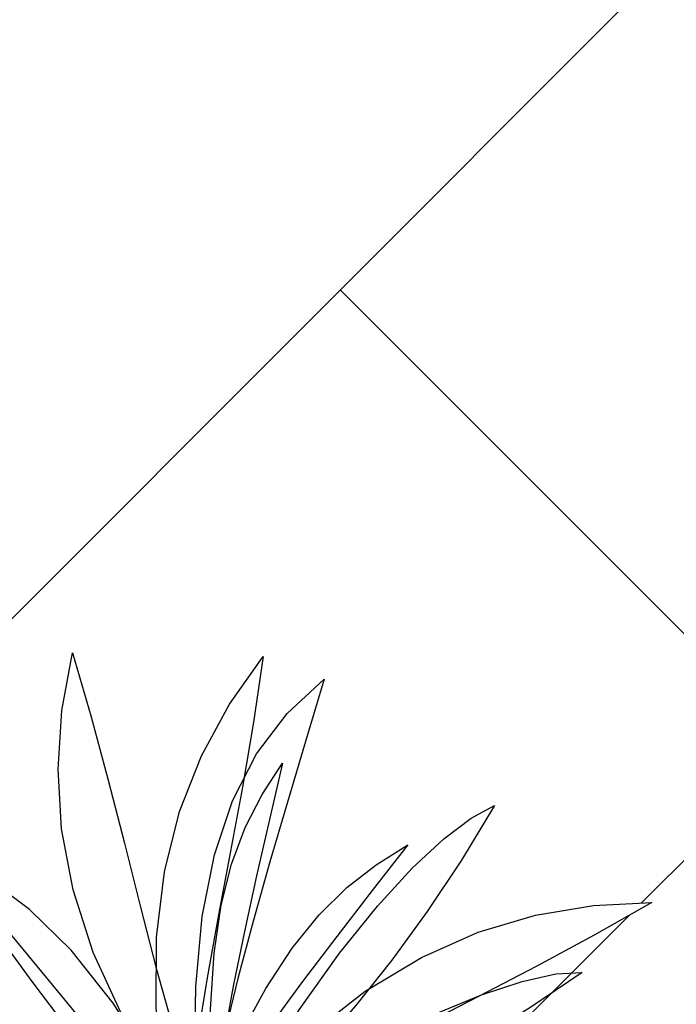
# Model space of a CAD drawing. Units: inches. Extents: x 3590 to 5167, y 65 to 1917.
# Tile 34 of 100: x 4947 to 4968, y 1357 to 1388. Entities that reach past the tile are written whole.
import ezdxf

# ---------------------------------------------------------------- set-up
doc = ezdxf.new("R2010")
doc.units = ezdxf.units.IN
doc.layers.add('A-FLOR-PATT', color=8, linetype='Continuous', lineweight=13)
doc.layers.add('L-PLNT', color=94, linetype='Continuous', lineweight=18)
doc.layers.add('DIENHOA', color=3, linetype='Continuous')

# ---------------------------------------------------------------- blocks, each defined once
blk = doc.blocks.new('Cay03_mb')
at = {"layer": 'DIENHOA'}
for p, q in [((118.6, 555.3), (166.2, 599.1)), ((166.2, 599.1), (142.2, 519.4)), ((79.5, 503.7), (118.6, 555.3)), ((142.2, 519.4), (119, 441.7)), ((48.6, 443.6), (79.5, 503.7)), ((25.5, 374.3), (48.6, 443.6)), ((119, 441.7), (96.7, 365.6)), ((9.9, 295.3), (25.5, 374.3)), ((96.7, 365.6), (75.6, 290.6)), ((-211.2, 304.6), (-263.5, 343.5)), ((-158, 252.3), (-211.2, 304.6)), ((436.8, 297.2), (511, 309.6)), ((511, 309.6), (585.9, 313.5)), ((585.9, 313.5), (511.8, 271.4)), ((1.6, 205.7), (9.9, 295.3)), ((75.6, 290.6), (55.7, 216.3)), ((363.4, 275.4), (436.8, 297.2)), ((-240.2, 277.8), (-88.4, 94.9)), ((290.6, 243.2), (363.4, 275.4)), ((511.8, 271.4), (437.6, 231.5)), ((-104.2, 184.4), (-158, 252.3)), ((218.5, 199.8), (290.6, 243.2)), ((437.6, 231.5), (363.7, 192.9)), ((55.7, 216.3), (37.3, 142.1)), ((0.2, 104.9), (1.6, 205.7)), ((147, 144.1), (218.5, 199.8)), ((363.7, 192.9), (290.2, 154.9)), ((-49.6, 98.5), (-104.2, 184.4))]:
    blk.add_line(p, q, dxfattribs=at)
for points in [[(23.7, -5.4), (-41, 82.2), (-91.8, 167.1), (-129.7, 249.5), (-155.6, 329.6), (-170.2, 407.8), (-174.7, 484.2), (-169.8, 559.3), (-156.5, 633.1)], [(-156.5, 633.1), (-132.5, 551.3), (-110.5, 470), (-89.8, 389.2), (-69.6, 309), (-49, 229.4), (-27.1, 150.4), (-3.2, 72.1), (23.7, -5.4)], [(-16.4, -26.7), (-38.3, 80), (-48.9, 178.3), (-48.7, 269), (-38.5, 352.6), (-19.1, 429.7), (9, 501), (44.9, 567.1), (87.9, 628.5)], [(87.9, 628.5), (75.5, 544.2), (61.3, 461.2), (46.1, 379.1), (30.8, 297.8), (16.1, 216.9), (2.9, 136), (-8.3, 54.9), (-16.4, -26.7)], [(23.7, -5.4), (19.8, 93), (20.3, 177), (25, 248.5), (34, 309.8), (47.3, 362.7), (64.9, 409.3), (86.8, 451.7), (112.9, 491.9)], [(112.9, 491.9), (96, 419.7), (79.5, 347.4), (63.9, 276.5), (50, 208.4), (38.4, 144.8), (29.7, 86.9), (24.6, 36.3), (23.7, -5.4)], [(-395.6, 473.7), (-347.5, 405.6), (-300.6, 339.5), (-254.3, 275.1), (-208.3, 212.3), (-161.9, 150.9), (-114.8, 90.7), (-66.5, 31.6), (-16.4, -26.7)], [(384.3, 437.5), (342.2, 367.8), (298.1, 301.7), (252.6, 239.4), (206.1, 181.1), (159.4, 127.2), (113, 78), (67.6, 33.6), (23.7, -5.4)], [(23.7, -5.4), (79.9, 91.7), (134.1, 176.2), (185.8, 248.4), (234.3, 308.7), (279, 357.3), (319.3, 394.8), (354.6, 421.4), (384.3, 437.5)], [(273.2, 387.3), (227.6, 328.8), (182.3, 270.1), (138.4, 212.3), (97.2, 156.4), (60, 103.4), (27.8, 54.6), (1.9, 10.8), (-16.4, -26.7)], [(-16.4, -26.7), (21.4, 64.2), (57, 140.3), (91.4, 203.3), (125.2, 255.1), (159.5, 297.5), (195, 332.5), (232.7, 361.8), (273.2, 387.3)], [(496.7, 224), (429.4, 178.4), (361.6, 136.9), (294.1, 99.5), (227.5, 66.1), (162.4, 36.7), (99.7, 11.5), (39.8, -9.7), (-16.4, -26.7)], [(-16.4, -26.7), (75.4, 37.9), (160.1, 91.8), (237.3, 135.7), (306.6, 170), (367.6, 195.4), (419.9, 212.5), (463.1, 221.9), (496.7, 224)]]:
    blk.add_lwpolyline(points, dxfattribs=at)

msp = doc.modelspace()

# ---------------------------------------------------------------- hatches: boundary and pattern name
at = {"layer": 'A-FLOR-PATT', "transparency": 33554687}
h = msp.add_hatch(dxfattribs=at)
h.set_pattern_fill('AR-HBONE', color=256, scale=0.2)
h.set_pattern_definition([(45, (-588.972, 0), (0, 28.73682), [60.96, -20.32]), (135, (-574.604, 14.368), (3e-15, 28.73682), [60.96, -20.32])])
h.paths.add_polyline_path([(5071.274, 1796.999), (4933.274, 1796.999), (4933.274, 1753.999), (4962.774, 1753.999, -0.414214), (4928.774, 1719.999), (4933.274, 1718.999), (4933.274, 1334.999), (5071.274, 1334.999)])
h.paths.add_polyline_path([(4951.78, 1521.077), (4951.715, 1521.04), (4951.563, 1520.895)], flags=16)
h.paths.add_polyline_path([(4952.267, 1521.376), (4952.198, 1521.371), (4952.198, 1521.356)], flags=0)
h.paths.add_polyline_path([(4967.051, 1529.728), (4965.231, 1528.694), (4963.411, 1527.714), (4961.756, 1526.851), (4963.589, 1527.449), (4964.036, 1527.478), (4962.975, 1527.249), (4961.76, 1526.852), (4959.792, 1525.834), (4958.005, 1524.895), (4956.24, 1523.93), (4954.504, 1522.919), (4954.129, 1522.682), (4953.361, 1521.997), (4953.366, 1521.998), (4953.605, 1522.064), (4955.106, 1522.761), (4956.921, 1523.434), (4958.678, 1523.915), (4960.358, 1524.2), (4961.945, 1524.286), (4964.171, 1524.108), (4965.958, 1523.309), (4963.863, 1522.976), (4965.187, 1522.499), (4963.366, 1522.497), (4961.545, 1522.487), (4959.764, 1522.461), (4958.304, 1522.419), (4957.974, 1522.388), (4956.307, 1522.232), (4954.718, 1522.071), (4953.251, 1521.899), (4953.525, 1521.623), (4954.331, 1521.379), (4956.243, 1521.23), (4958.039, 1520.93), (4959.684, 1520.483), (4961.16, 1519.896), (4963.107, 1518.8), (4964.393, 1517.325), (4962.973, 1517.726), (4964.558, 1516.661), (4965.407, 1515.708), (4963.507, 1516.322), (4961.68, 1517.005), (4959.935, 1517.745), (4958.282, 1518.528), (4956.732, 1519.343), (4955.295, 1520.175), (4954.672, 1520.572), (4954.513, 1520.627), (4955.658, 1519.318), (4956.703, 1517.982), (4957.644, 1516.647), (4958.485, 1515.334), (4959.55, 1513.524), (4960.438, 1511.769), (4958.841, 1513.62), (4957.452, 1515.325), (4955.819, 1517.459), (4956.665, 1515.448), (4957.111, 1513.923), (4957.447, 1511.714), (4957.076, 1509.793), (4956.538, 1511.11), (4955.992, 1512.569), (4955.444, 1514.125), (4954.898, 1515.735), (4954.357, 1517.356), (4953.824, 1518.943), (4953.305, 1520.452), (4953.065, 1521.116), (4952.971, 1521.146), (4952.949, 1521.086), (4952.73, 1520.199), (4953.37, 1518.024), (4953.757, 1516.373), (4954.051, 1514.765), (4954.264, 1513.221), (4954.471, 1511.131), (4954.497, 1510.402), (4954.409, 1511.76), (4954.264, 1513.221), (4954.051, 1514.765), (4953.757, 1516.373), (4953.37, 1518.024), (4952.877, 1519.698), (4952.716, 1520.141), (4952.533, 1519.059), (4952.374, 1517.789), (4952.219, 1516.312), (4952.046, 1514.6), (4951.833, 1512.626), (4951.557, 1510.363), (4951.203, 1512.168), (4950.852, 1514.339), (4950.985, 1516.376), (4951.66, 1518.286), (4952.593, 1520.481), (4952.357, 1521.13), (4951.855, 1520.328), (4950.839, 1518.908), (4949.777, 1517.587), (4948.916, 1516.617), (4948.111, 1515.256), (4947.089, 1513.554), (4945.889, 1511.615), (4946.326, 1513.402), (4946.562, 1514.249), (4945.528, 1513.327), (4944.581, 1512.531), (4946.018, 1514.508), (4947.204, 1516.048), (4947.893, 1517.313), (4949.307, 1518.764), (4950.414, 1519.767), (4950.451, 1519.806), (4952.267, 1521.376), (4951.645, 1521.493), (4950.404, 1521.18), (4948.044, 1520.359), (4946.119, 1519.452), (4944.572, 1518.475), (4943.35, 1517.443), (4941.997, 1515.92), (4941.661, 1515.275), (4942.813, 1516.99), (4944.572, 1518.475), (4946.119, 1519.452), (4948.044, 1520.359), (4950.404, 1521.18), (4951.645, 1521.493), (4949.647, 1521.868), (4948.6, 1521.756), (4947.126, 1521.57), (4945.42, 1521.348), (4943.45, 1521.105), (4941.183, 1520.856), (4942.86, 1521.613), (4943.873, 1522.03), (4942.952, 1521.909), (4941.41, 1521.485), (4939.543, 1520.67), (4938.968, 1520.226), (4940.733, 1521.299), (4942.952, 1521.909), (4943.702, 1522.008), (4945.894, 1522.7), (4947.565, 1522.714), (4948.921, 1522.566), (4951.131, 1522.183), (4950.971, 1522.297), (4948.129, 1523.006), (4946.035, 1523.707), (4944.232, 1524.521), (4942.707, 1525.461), (4941.444, 1526.537), (4940.43, 1527.761), (4939.649, 1529.143), (4941.421, 1528.122), (4943.147, 1527.132), (4944.841, 1526.175), (4946.514, 1525.25), (4948.179, 1524.359), (4948.365, 1524.263), (4946.475, 1526.045), (4945.181, 1527.54), (4944.19, 1529.033), (4943.496, 1530.54), (4943.278, 1531.36), (4942.498, 1531.919), (4943.114, 1531.762), (4942.959, 1533.659), (4944.14, 1531.989), (4944.612, 1531.323), (4946.202, 1530.463), (4947.486, 1529.509), (4948.79, 1528.226), (4950.368, 1526.237), (4949.485, 1528.155), (4948.851, 1530.123), (4948.491, 1532.041), (4948.381, 1533.918), (4948.501, 1535.76), (4948.827, 1537.573), (4949.418, 1535.565), (4949.957, 1533.569), (4950.464, 1531.586), (4950.961, 1529.617), (4951.391, 1527.954), (4951.724, 1530.687), (4952.201, 1532.58), (4952.889, 1534.33), (4953.77, 1535.951), (4954.827, 1537.46), (4954.521, 1535.39), (4954.273, 1533.937), (4955.58, 1535.663), (4956.748, 1536.739), (4956.159, 1534.78), (4955.589, 1532.873), (4955.043, 1531.006), (4954.525, 1529.166), (4954.038, 1527.341), (4953.638, 1525.733), (4953.611, 1525.586), (4953.398, 1524.166), (4953.382, 1524.009), (4954.07, 1525.476), (4954.912, 1527.022), (4956.136, 1528.894), (4957.847, 1530.577), (4959.376, 1531.54), (4958.256, 1530.104), (4957.143, 1528.663), (4956.066, 1527.243), (4955.056, 1525.871), (4954.141, 1524.571), (4953.352, 1523.372), (4953.311, 1523.303), (4953.273, 1522.925), (4953.261, 1522.382), (4954.103, 1523.373), (4954.63, 1524.284), (4955.961, 1526.358), (4957.23, 1528.13), (4958.421, 1529.609), (4960.037, 1531.368), (4961.374, 1532.375), (4962.101, 1532.77), (4961.07, 1531.061), (4959.987, 1529.438), (4958.869, 1527.908), (4958.15, 1527.007), (4959.803, 1528.003), (4961.589, 1528.793), (4963.391, 1529.328), (4965.211, 1529.632)], flags=16)
h.paths.add_polyline_path([(4962.944, 1523.182), (4961.107, 1523.422), (4960.392, 1523.362), (4962.35, 1523.331)], flags=0)
h.paths.add_polyline_path([(5049.541, 1584.551), (5049.476, 1584.515), (5049.325, 1584.37)], flags=16)
h.paths.add_polyline_path([(5050.028, 1584.851), (5049.959, 1584.845), (5049.959, 1584.83)], flags=0)
h.paths.add_polyline_path([(5042.333, 1581.949), (5043.88, 1582.926), (5045.806, 1583.833), (5048.165, 1584.654), (5049.406, 1584.967), (5047.408, 1585.342), (5046.361, 1585.231), (5044.888, 1585.044), (5043.181, 1584.822), (5041.211, 1584.579), (5038.944, 1584.33), (5040.622, 1585.087), (5041.634, 1585.504), (5040.713, 1585.383), (5039.171, 1584.959), (5037.304, 1584.144), (5036.729, 1583.7), (5038.494, 1584.773), (5040.713, 1585.383), (5041.463, 1585.482), (5043.655, 1586.174), (5045.326, 1586.188), (5046.682, 1586.04), (5048.893, 1585.657), (5048.732, 1585.771), (5045.891, 1586.48), (5043.796, 1587.181), (5041.994, 1587.996), (5040.468, 1588.935), (5039.205, 1590.011), (5038.191, 1591.235), (5037.41, 1592.617), (5039.182, 1591.596), (5040.909, 1590.607), (5042.602, 1589.649), (5044.275, 1588.724), (5045.94, 1587.833), (5046.126, 1587.738), (5044.237, 1589.519), (5042.942, 1591.015), (5041.952, 1592.508), (5041.257, 1594.014), (5041.039, 1594.834), (5040.26, 1595.393), (5040.875, 1595.237), (5040.721, 1597.133), (5041.901, 1595.463), (5042.373, 1594.798), (5043.963, 1593.938), (5045.247, 1592.983), (5046.552, 1591.701), (5048.129, 1589.712), (5047.247, 1591.63), (5046.613, 1593.597), (5046.252, 1595.515), (5046.142, 1597.392), (5046.262, 1599.234), (5046.588, 1601.047), (5047.179, 1599.039), (5047.718, 1597.043), (5048.225, 1595.06), (5048.722, 1593.091), (5049.152, 1591.429), (5049.485, 1594.161), (5049.962, 1596.054), (5050.65, 1597.804), (5051.532, 1599.425), (5052.589, 1600.934), (5052.283, 1598.864), (5052.034, 1597.411), (5053.341, 1599.137), (5054.509, 1600.213), (5053.92, 1598.254), (5053.35, 1596.348), (5052.805, 1594.48), (5052.286, 1592.64), (5051.799, 1590.815), (5051.4, 1589.207), (5051.373, 1589.06), (5051.159, 1587.64), (5051.143, 1587.483), (5051.831, 1588.95), (5052.673, 1590.496), (5053.898, 1592.368), (5055.608, 1594.051), (5057.137, 1595.014), (5056.017, 1593.578), (5054.904, 1592.137), (5053.828, 1590.717), (5052.817, 1589.345), (5051.902, 1588.046), (5051.113, 1586.846), (5051.072, 1586.777), (5051.034, 1586.399), (5051.022, 1585.856), (5051.864, 1586.847), (5052.391, 1587.758), (5053.723, 1589.832), (5054.991, 1591.604), (5056.182, 1593.083), (5057.798, 1594.842), (5059.135, 1595.849), (5059.863, 1596.244), (5058.831, 1594.535), (5057.749, 1592.912), (5056.63, 1591.382), (5055.912, 1590.482), (5057.564, 1591.477), (5059.35, 1592.267), (5061.152, 1592.802), (5062.972, 1593.106), (5064.812, 1593.203), (5062.992, 1592.169), (5061.172, 1591.188), (5059.518, 1590.325), (5061.35, 1590.924), (5061.797, 1590.952), (5060.737, 1590.723), (5059.521, 1590.326), (5057.553, 1589.308), (5055.766, 1588.369), (5054.002, 1587.404), (5052.265, 1586.393), (5051.891, 1586.156), (5051.122, 1585.471), (5051.127, 1585.472), (5051.366, 1585.538), (5052.867, 1586.235), (5054.682, 1586.908), (5056.439, 1587.389), (5058.12, 1587.675), (5059.706, 1587.76), (5061.933, 1587.583), (5063.719, 1586.783), (5061.624, 1586.45), (5062.949, 1585.973), (5061.127, 1585.971), (5059.307, 1585.961), (5057.525, 1585.935), (5056.065, 1585.893), (5055.735, 1585.862), (5054.068, 1585.707), (5052.479, 1585.546), (5051.012, 1585.373), (5051.286, 1585.097), (5052.092, 1584.853), (5054.004, 1584.704), (5055.8, 1584.404), (5057.446, 1583.958), (5058.921, 1583.37), (5060.868, 1582.274), (5062.154, 1580.799), (5060.734, 1581.2), (5062.32, 1580.135), (5063.168, 1579.182), (5061.269, 1579.796), (5059.441, 1580.479), (5057.696, 1581.219), (5056.043, 1582.003), (5054.493, 1582.817), (5053.057, 1583.649), (5052.433, 1584.047), (5052.274, 1584.101), (5053.42, 1582.793), (5054.464, 1581.457), (5055.405, 1580.121), (5056.247, 1578.809), (5057.311, 1576.998), (5058.199, 1575.244), (5056.602, 1577.094), (5055.213, 1578.799), (5053.58, 1580.933), (5054.427, 1578.922), (5054.872, 1577.397), (5055.208, 1575.189), (5054.838, 1573.267), (5054.299, 1574.584), (5053.754, 1576.043), (5053.206, 1577.599), (5052.659, 1579.209), (5052.118, 1580.83), (5051.585, 1582.417), (5051.066, 1583.927), (5050.826, 1584.59), (5050.733, 1584.62), (5050.711, 1584.561), (5050.491, 1583.673), (5051.131, 1581.498), (5051.518, 1579.847), (5051.813, 1578.24), (5052.026, 1576.695), (5052.233, 1574.605), (5052.258, 1573.876), (5052.17, 1575.234), (5052.026, 1576.695), (5051.813, 1578.24), (5051.518, 1579.847), (5051.131, 1581.498), (5050.638, 1583.172), (5050.477, 1583.615), (5050.294, 1582.533), (5050.136, 1581.263), (5049.981, 1579.786), (5049.807, 1578.074), (5049.594, 1576.1), (5049.318, 1573.837), (5048.965, 1575.642), (5048.613, 1577.813), (5048.747, 1579.85), (5049.421, 1581.76), (5050.354, 1583.955), (5050.118, 1584.604), (5049.616, 1583.802), (5048.6, 1582.382), (5047.538, 1581.061), (5046.677, 1580.091), (5045.872, 1578.73), (5044.85, 1577.028), (5043.651, 1575.089), (5044.087, 1576.877), (5044.324, 1577.723), (5043.289, 1576.801), (5042.342, 1576.005), (5043.779, 1577.982), (5044.966, 1579.522), (5045.655, 1580.787), (5047.068, 1582.239), (5048.175, 1583.241), (5048.213, 1583.28), (5050.028, 1584.851), (5049.406, 1584.967), (5048.165, 1584.654), (5045.806, 1583.833), (5043.88, 1582.926), (5042.333, 1581.949), (5041.111, 1580.917), (5039.758, 1579.394), (5039.423, 1578.749), (5040.575, 1580.464)], flags=16)
h.paths.add_polyline_path([(4954.799, 1533.12), (4954.262, 1532.079), (4953.831, 1530.935), (4953.505, 1529.636), (4953.283, 1528.133), (4953.167, 1526.376), (4953.156, 1524.315), (4953.277, 1521.236), (4952.802, 1521.842), (4951.557, 1521.998), (4950.976, 1521.961), (4952.661, 1521.941), (4952.802, 1521.842), (4953.152, 1523.593), (4953.167, 1526.376), (4953.283, 1528.133), (4953.609, 1530.346), (4954.456, 1532.592)], flags=0)
h.paths.add_polyline_path([(5050.563, 1585.316), (5049.318, 1585.472), (5048.737, 1585.435), (5050.422, 1585.415), (5050.563, 1585.316), (5050.914, 1587.067), (5050.928, 1589.851), (5051.045, 1591.607), (5051.371, 1593.82), (5052.217, 1596.066), (5052.56, 1596.594), (5052.024, 1595.554), (5051.592, 1594.409), (5051.266, 1593.11), (5051.045, 1591.607), (5050.928, 1589.851), (5050.918, 1587.789), (5051.038, 1584.71)], flags=0)
h.paths.add_polyline_path([(5058.153, 1586.836), (5060.111, 1586.805), (5060.705, 1586.656), (5058.868, 1586.896)], flags=0)
h.paths.add_polyline_path([(5049.541, 1430.936), (5049.476, 1430.9), (5049.325, 1430.755)], flags=16)
h.paths.add_polyline_path([(5050.028, 1431.236), (5049.959, 1431.231), (5049.959, 1431.215)], flags=0)
h.paths.add_polyline_path([(5046.588, 1447.432), (5047.179, 1445.425), (5047.718, 1443.429), (5048.225, 1441.446), (5048.722, 1439.476), (5049.152, 1437.814), (5049.485, 1440.546), (5049.962, 1442.439), (5050.65, 1444.189), (5051.532, 1445.811), (5052.589, 1447.319), (5052.283, 1445.249), (5052.034, 1443.796), (5053.341, 1445.522), (5054.509, 1446.598), (5053.92, 1444.64), (5053.35, 1442.733), (5052.805, 1440.865), (5052.286, 1439.025), (5051.799, 1437.201), (5051.4, 1435.592), (5051.373, 1435.445), (5051.159, 1434.025), (5051.143, 1433.868), (5051.831, 1435.335), (5052.673, 1436.881), (5053.898, 1438.753), (5055.608, 1440.436), (5057.137, 1441.4), (5056.017, 1439.963), (5054.904, 1438.522), (5053.828, 1437.102), (5052.817, 1435.73), (5051.902, 1434.431), (5051.113, 1433.231), (5051.072, 1433.162), (5051.034, 1432.784), (5051.022, 1432.242), (5051.864, 1433.232), (5052.391, 1434.143), (5053.723, 1436.217), (5054.991, 1437.989), (5056.182, 1439.468), (5057.798, 1441.227), (5059.135, 1442.235), (5059.863, 1442.629), (5058.831, 1440.921), (5057.749, 1439.298), (5056.63, 1437.767), (5055.912, 1436.867), (5057.564, 1437.863), (5059.35, 1438.652), (5061.152, 1439.187), (5062.972, 1439.491), (5064.812, 1439.588), (5062.992, 1438.554), (5061.172, 1437.573), (5059.518, 1436.71), (5061.35, 1437.309), (5061.797, 1437.337), (5060.737, 1437.108), (5059.521, 1436.711), (5057.553, 1435.693), (5055.766, 1434.754), (5054.002, 1433.789), (5052.265, 1432.778), (5051.891, 1432.541), (5051.122, 1431.856), (5051.127, 1431.857), (5051.366, 1431.923), (5052.867, 1432.62), (5054.682, 1433.293), (5056.439, 1433.775), (5058.12, 1434.06), (5059.706, 1434.145), (5061.933, 1433.968), (5063.719, 1433.168), (5061.624, 1432.835), (5062.949, 1432.358), (5061.127, 1432.357), (5059.307, 1432.346), (5057.525, 1432.32), (5056.065, 1432.278), (5055.735, 1432.248), (5054.068, 1432.092), (5052.479, 1431.931), (5051.012, 1431.759), (5051.286, 1431.482), (5052.092, 1431.238), (5054.004, 1431.089), (5055.8, 1430.789), (5057.446, 1430.343), (5058.921, 1429.755), (5060.868, 1428.66), (5062.154, 1427.185), (5060.734, 1427.585), (5062.32, 1426.52), (5063.168, 1425.567), (5061.269, 1426.181), (5059.441, 1426.865), (5057.696, 1427.604), (5056.043, 1428.388), (5054.493, 1429.202), (5053.057, 1430.034), (5052.433, 1430.432), (5052.274, 1430.487), (5053.42, 1429.178), (5054.464, 1427.842), (5055.405, 1426.506), (5056.247, 1425.194), (5057.311, 1423.383), (5058.199, 1421.629), (5056.602, 1423.479), (5055.213, 1425.184), (5053.58, 1427.318), (5054.427, 1425.307), (5054.872, 1423.782), (5055.208, 1421.574), (5054.838, 1419.652), (5054.299, 1420.97), (5053.754, 1422.428), (5053.206, 1423.984), (5052.659, 1425.595), (5052.118, 1427.215), (5051.585, 1428.802), (5051.066, 1430.312), (5050.826, 1430.975), (5050.733, 1431.005), (5050.711, 1430.946), (5050.491, 1430.058), (5051.131, 1427.883), (5051.518, 1426.232), (5051.813, 1424.625), (5052.026, 1423.081), (5052.233, 1420.991), (5052.258, 1420.261), (5052.17, 1421.619), (5052.026, 1423.081), (5051.813, 1424.625), (5051.518, 1426.232), (5051.131, 1427.883), (5050.638, 1429.558), (5050.477, 1430.001), (5050.294, 1428.918), (5050.136, 1427.648), (5049.981, 1426.171), (5049.807, 1424.459), (5049.594, 1422.485), (5049.318, 1420.222), (5048.965, 1422.028), (5048.613, 1424.199), (5048.747, 1426.235), (5049.421, 1428.146), (5050.354, 1430.34), (5050.118, 1430.989), (5049.616, 1430.187), (5048.6, 1428.768), (5047.538, 1427.446), (5046.677, 1426.477), (5045.872, 1425.116), (5044.85, 1423.413), (5043.651, 1421.474), (5044.087, 1423.262), (5044.324, 1424.109), (5043.289, 1423.186), (5042.342, 1422.391), (5043.779, 1424.368), (5044.966, 1425.907), (5045.655, 1427.173), (5047.068, 1428.624), (5048.175, 1429.627), (5048.213, 1429.666), (5050.028, 1431.236), (5049.406, 1431.353), (5048.165, 1431.039), (5045.806, 1430.218), (5043.88, 1429.311), (5042.333, 1428.334), (5041.111, 1427.302), (5039.758, 1425.779), (5039.423, 1425.134), (5040.575, 1426.849), (5042.333, 1428.334), (5043.88, 1429.311), (5045.806, 1430.218), (5048.165, 1431.039), (5049.406, 1431.353), (5047.408, 1431.727), (5046.361, 1431.616), (5044.888, 1431.429), (5043.181, 1431.207), (5041.211, 1430.964), (5038.944, 1430.715), (5040.622, 1431.472), (5041.634, 1431.89), (5040.713, 1431.769), (5039.171, 1431.345), (5037.304, 1430.53), (5036.729, 1430.085), (5038.494, 1431.158), (5040.713, 1431.769), (5041.463, 1431.867), (5043.655, 1432.559), (5045.326, 1432.573), (5046.682, 1432.425), (5048.893, 1432.042), (5048.732, 1432.156), (5045.891, 1432.865), (5043.796, 1433.566), (5041.994, 1434.381), (5040.468, 1435.321), (5039.205, 1436.396), (5038.191, 1437.62), (5037.41, 1439.002), (5039.182, 1437.982), (5040.909, 1436.992), (5042.602, 1436.034), (5044.275, 1435.109), (5045.94, 1434.218), (5046.126, 1434.123), (5044.237, 1435.904), (5042.942, 1437.4), (5041.952, 1438.893), (5041.257, 1440.399), (5041.039, 1441.219), (5040.26, 1441.778), (5040.875, 1441.622), (5040.721, 1443.518), (5041.901, 1441.848), (5042.373, 1441.183), (5043.963, 1440.323), (5045.247, 1439.369), (5046.552, 1438.086), (5048.129, 1436.097), (5047.247, 1438.015), (5046.613, 1439.982), (5046.252, 1441.901), (5046.142, 1443.778), (5046.262, 1445.619)], flags=16)
h.paths.add_polyline_path([(5052.382, 1444.255), (5051.623, 1442.78), (5052.024, 1441.939), (5052.56, 1442.98)], flags=0)
h.paths.add_polyline_path([(5050.563, 1431.701), (5049.318, 1431.857), (5048.737, 1431.821), (5050.422, 1431.8)], flags=0)
h.paths.add_polyline_path([(5058.153, 1433.221), (5060.111, 1433.19), (5060.705, 1433.041), (5058.868, 1433.281)], flags=0)
h.paths.add_polyline_path([(5049.541, 1352.285), (5049.476, 1352.249), (5049.325, 1352.104)], flags=16)
h.paths.add_polyline_path([(5050.028, 1352.585), (5049.959, 1352.58), (5049.959, 1352.564)], flags=0)
h.paths.add_polyline_path([(5046.588, 1368.781), (5047.179, 1366.774), (5047.718, 1364.778), (5048.225, 1362.795), (5048.722, 1360.825), (5049.152, 1359.163), (5049.485, 1361.896), (5049.962, 1363.789), (5050.65, 1365.538), (5051.532, 1367.16), (5052.589, 1368.669), (5052.283, 1366.598), (5052.034, 1365.145), (5053.341, 1366.871), (5054.509, 1367.947), (5053.92, 1365.989), (5053.35, 1364.082), (5052.805, 1362.214), (5052.286, 1360.374), (5051.799, 1358.55), (5051.4, 1356.942), (5051.373, 1356.794), (5051.159, 1355.374), (5051.143, 1355.218), (5051.831, 1356.684), (5052.673, 1358.23), (5053.898, 1360.102), (5055.608, 1361.786), (5057.137, 1362.749), (5056.017, 1361.313), (5054.904, 1359.872), (5053.828, 1358.452), (5052.817, 1357.079), (5051.902, 1355.78), (5051.113, 1354.581), (5051.072, 1354.512), (5051.034, 1354.133), (5051.022, 1353.591), (5051.864, 1354.581), (5052.391, 1355.492), (5053.723, 1357.566), (5054.991, 1359.338), (5056.182, 1360.817), (5057.798, 1362.577), (5059.135, 1363.584), (5059.863, 1363.979), (5058.831, 1362.27), (5057.749, 1360.647), (5056.63, 1359.117), (5055.912, 1358.216), (5057.564, 1359.212), (5059.35, 1360.001), (5061.152, 1360.536), (5062.972, 1360.841), (5064.812, 1360.937), (5062.992, 1359.903), (5061.172, 1358.923), (5059.518, 1358.059), (5061.35, 1358.658), (5061.797, 1358.687), (5060.737, 1358.458), (5059.521, 1358.061), (5057.553, 1357.043), (5055.766, 1356.103), (5054.002, 1355.138), (5052.265, 1354.127), (5051.891, 1353.89), (5051.122, 1353.206), (5051.127, 1353.206), (5051.366, 1353.272), (5052.867, 1353.969), (5054.682, 1354.643), (5056.439, 1355.124), (5058.12, 1355.409), (5059.706, 1355.495), (5061.933, 1355.317), (5063.719, 1354.518), (5061.624, 1354.184), (5062.949, 1353.708), (5061.127, 1353.706), (5059.307, 1353.695), (5057.525, 1353.669), (5056.065, 1353.627), (5055.735, 1353.597), (5054.068, 1353.441), (5052.479, 1353.28), (5051.012, 1353.108), (5051.286, 1352.831), (5052.092, 1352.587), (5054.004, 1352.439), (5055.8, 1352.138), (5057.446, 1351.692), (5058.921, 1351.104), (5060.868, 1350.009), (5062.154, 1348.534), (5060.734, 1348.935), (5062.32, 1347.869), (5063.168, 1346.916), (5061.269, 1347.53), (5059.441, 1348.214), (5057.696, 1348.954), (5056.043, 1349.737), (5054.493, 1350.551), (5053.057, 1351.383), (5052.433, 1351.781), (5052.274, 1351.836), (5053.42, 1350.527), (5054.464, 1349.191), (5055.405, 1347.855), (5056.247, 1346.543), (5057.311, 1344.733), (5058.199, 1342.978), (5056.602, 1344.828), (5055.213, 1346.534), (5053.58, 1348.667), (5054.427, 1346.656), (5054.872, 1345.132), (5055.208, 1342.923), (5054.838, 1341.002), (5054.299, 1342.319), (5053.754, 1343.778), (5053.206, 1345.334), (5052.659, 1346.944), (5052.118, 1348.564), (5051.585, 1350.151), (5051.066, 1351.661), (5050.826, 1352.324), (5050.733, 1352.355), (5050.711, 1352.295), (5050.491, 1351.408), (5051.131, 1349.232), (5051.518, 1347.581), (5051.813, 1345.974), (5052.026, 1344.43), (5052.233, 1342.34), (5052.258, 1341.61), (5052.17, 1342.969), (5052.026, 1344.43), (5051.813, 1345.974), (5051.518, 1347.581), (5051.131, 1349.232), (5050.638, 1350.907), (5050.477, 1351.35), (5050.294, 1350.267), (5050.136, 1348.997), (5049.981, 1347.52), (5049.807, 1345.809), (5049.594, 1343.835), (5049.318, 1341.571), (5048.965, 1343.377), (5048.613, 1345.548), (5048.747, 1347.585), (5049.421, 1349.495), (5050.354, 1351.689), (5050.118, 1352.339), (5049.616, 1351.536), (5048.6, 1350.117), (5047.538, 1348.795), (5046.677, 1347.826), (5045.872, 1346.465), (5044.85, 1344.763), (5043.651, 1342.824), (5044.087, 1344.611), (5044.324, 1345.458), (5043.289, 1344.535), (5042.342, 1343.74), (5043.779, 1345.717), (5044.966, 1347.256), (5045.655, 1348.522), (5047.068, 1349.973), (5048.175, 1350.976), (5048.213, 1351.015), (5050.028, 1352.585), (5049.406, 1352.702), (5048.165, 1352.388), (5045.806, 1351.567), (5043.88, 1350.661), (5042.333, 1349.683), (5041.111, 1348.651), (5039.758, 1347.128), (5039.423, 1346.483), (5040.575, 1348.198), (5042.333, 1349.683), (5043.88, 1350.661), (5045.806, 1351.567), (5048.165, 1352.388), (5049.406, 1352.702), (5047.408, 1353.076), (5046.361, 1352.965), (5044.888, 1352.779), (5043.181, 1352.556), (5041.211, 1352.313), (5038.944, 1352.065), (5040.622, 1352.821), (5041.634, 1353.239), (5040.713, 1353.118), (5039.171, 1352.694), (5037.304, 1351.879), (5036.729, 1351.434), (5038.494, 1352.508), (5040.713, 1353.118), (5041.463, 1353.216), (5043.655, 1353.909), (5045.326, 1353.923), (5046.682, 1353.774), (5048.893, 1353.391), (5048.732, 1353.506), (5045.891, 1354.214), (5043.796, 1354.915), (5041.994, 1355.73), (5040.468, 1356.67), (5039.205, 1357.746), (5038.191, 1358.969), (5037.41, 1360.352), (5039.182, 1359.331), (5040.909, 1358.341), (5042.602, 1357.383), (5044.275, 1356.458), (5045.94, 1355.567), (5046.126, 1355.472), (5044.237, 1357.253), (5042.942, 1358.749), (5041.952, 1360.242), (5041.257, 1361.748), (5041.039, 1362.568), (5040.26, 1363.128), (5040.875, 1362.971), (5040.721, 1364.867), (5041.901, 1363.197), (5042.373, 1362.532), (5043.963, 1361.672), (5045.247, 1360.718), (5046.552, 1359.435), (5048.129, 1357.446), (5047.247, 1359.364), (5046.613, 1361.331), (5046.252, 1363.25), (5046.142, 1365.127), (5046.262, 1366.969)], flags=16)
h.paths.add_polyline_path([(5052.382, 1365.604), (5051.623, 1364.129), (5052.024, 1363.288), (5052.56, 1364.329)], flags=0)
h.paths.add_polyline_path([(4951.78, 1698.041), (4951.715, 1698.005), (4951.563, 1697.859)], flags=16)
h.paths.add_polyline_path([(4952.267, 1698.341), (4952.198, 1698.335), (4952.198, 1698.32)], flags=0)
h.paths.add_polyline_path([(4957.076, 1686.757), (4956.538, 1688.074), (4955.992, 1689.533), (4955.444, 1691.089), (4954.898, 1692.699), (4954.357, 1694.32), (4953.824, 1695.907), (4953.305, 1697.417), (4953.065, 1698.08), (4952.971, 1698.11), (4952.949, 1698.051), (4952.73, 1697.163), (4953.37, 1694.988), (4953.757, 1693.337), (4954.051, 1691.729), (4954.264, 1690.185), (4954.471, 1688.095), (4954.497, 1687.366), (4954.409, 1688.724), (4954.264, 1690.185), (4954.051, 1691.729), (4953.757, 1693.337), (4953.37, 1694.988), (4952.877, 1696.662), (4952.716, 1697.105), (4952.533, 1696.023), (4952.374, 1694.753), (4952.219, 1693.276), (4952.046, 1691.564), (4951.833, 1689.59), (4951.557, 1687.327), (4951.203, 1689.132), (4950.852, 1691.303), (4950.985, 1693.34), (4951.66, 1695.25), (4952.593, 1697.445), (4952.357, 1698.094), (4951.855, 1697.292), (4950.839, 1695.872), (4949.777, 1694.551), (4948.916, 1693.581), (4948.111, 1692.22), (4947.089, 1690.518), (4945.889, 1688.579), (4946.326, 1690.366), (4946.562, 1691.213), (4945.528, 1690.291), (4944.581, 1689.495), (4946.018, 1691.472), (4947.204, 1693.012), (4947.893, 1694.277), (4949.307, 1695.729), (4950.414, 1696.731), (4950.451, 1696.77), (4952.267, 1698.341), (4951.645, 1698.457), (4950.404, 1698.144), (4948.044, 1697.323), (4946.119, 1696.416), (4944.572, 1695.439), (4943.35, 1694.407), (4941.997, 1692.884), (4941.661, 1692.239), (4942.813, 1693.954), (4944.572, 1695.439), (4946.119, 1696.416), (4948.044, 1697.323), (4950.404, 1698.144), (4951.645, 1698.457), (4949.647, 1698.832), (4948.6, 1698.72), (4947.126, 1698.534), (4945.42, 1698.312), (4943.45, 1698.069), (4941.183, 1697.82), (4942.86, 1698.577), (4943.873, 1698.994), (4942.952, 1698.873), (4941.41, 1698.449), (4939.543, 1697.634), (4938.968, 1697.19), (4940.733, 1698.263), (4942.952, 1698.873), (4943.702, 1698.972), (4945.894, 1699.664), (4947.565, 1699.678), (4948.921, 1699.53), (4951.131, 1699.147), (4950.971, 1699.261), (4948.129, 1699.97), (4946.035, 1700.671), (4944.232, 1701.486), (4942.707, 1702.425), (4941.444, 1703.501), (4940.43, 1704.725), (4939.649, 1706.107), (4941.421, 1705.086), (4943.147, 1704.097), (4944.841, 1703.139), (4946.514, 1702.214), (4948.179, 1701.323), (4948.365, 1701.227), (4946.475, 1703.009), (4945.181, 1704.505), (4944.19, 1705.997), (4943.496, 1707.504), (4943.278, 1708.324), (4942.498, 1708.883), (4943.114, 1708.727), (4942.959, 1710.623), (4944.14, 1708.953), (4944.612, 1708.287), (4946.202, 1707.428), (4947.486, 1706.473), (4948.79, 1705.191), (4950.368, 1703.202), (4949.485, 1705.12), (4948.851, 1707.087), (4948.491, 1709.005), (4948.381, 1710.882), (4948.501, 1712.724), (4948.827, 1714.537), (4949.418, 1712.529), (4949.957, 1710.533), (4950.464, 1708.55), (4950.961, 1706.581), (4951.391, 1704.919), (4951.724, 1707.651), (4952.201, 1709.544), (4952.889, 1711.294), (4953.77, 1712.915), (4954.827, 1714.424), (4954.521, 1712.354), (4954.273, 1710.901), (4955.58, 1712.627), (4956.748, 1713.703), (4956.159, 1711.744), (4955.589, 1709.837), (4955.043, 1707.97), (4954.525, 1706.13), (4954.038, 1704.305), (4953.638, 1702.697), (4953.611, 1702.55), (4953.398, 1701.13), (4953.382, 1700.973), (4954.07, 1702.44), (4954.912, 1703.986), (4956.136, 1705.858), (4957.847, 1707.541), (4959.376, 1708.504), (4958.256, 1707.068), (4957.143, 1705.627), (4956.066, 1704.207), (4955.056, 1702.835), (4954.141, 1701.536), (4953.352, 1700.336), (4953.311, 1700.267), (4953.273, 1699.889), (4953.261, 1699.346), (4954.103, 1700.337), (4954.63, 1701.248), (4955.961, 1703.322), (4957.23, 1705.094), (4958.421, 1706.573), (4960.037, 1708.332), (4961.374, 1709.339), (4962.101, 1709.734), (4961.07, 1708.025), (4959.987, 1706.402), (4958.869, 1704.872), (4958.15, 1703.972), (4959.803, 1704.967), (4961.589, 1705.757), (4963.391, 1706.292), (4965.211, 1706.596), (4967.051, 1706.692), (4965.231, 1705.659), (4963.411, 1704.678), (4961.756, 1703.815), (4963.589, 1704.413), (4964.036, 1704.442), (4962.975, 1704.213), (4961.76, 1703.816), (4959.792, 1702.798), (4958.005, 1701.859), (4956.24, 1700.894), (4954.504, 1699.883), (4954.129, 1699.646), (4953.361, 1698.961), (4953.366, 1698.962), (4953.605, 1699.028), (4955.106, 1699.725), (4956.921, 1700.398), (4958.678, 1700.879), (4960.358, 1701.164), (4961.945, 1701.25), (4964.171, 1701.073), (4965.958, 1700.273), (4963.863, 1699.94), (4965.187, 1699.463), (4963.366, 1699.461), (4961.545, 1699.451), (4959.764, 1699.425), (4958.304, 1699.383), (4957.974, 1699.352), (4956.307, 1699.197), (4954.718, 1699.036), (4953.251, 1698.863), (4953.525, 1698.587), (4954.331, 1698.343), (4956.243, 1698.194), (4958.039, 1697.894), (4959.684, 1697.447), (4961.16, 1696.86), (4963.107, 1695.764), (4964.393, 1694.289), (4962.973, 1694.69), (4964.558, 1693.625), (4965.407, 1692.672), (4963.507, 1693.286), (4961.68, 1693.969), (4959.935, 1694.709), (4958.282, 1695.492), (4956.732, 1696.307), (4955.295, 1697.139), (4954.672, 1697.536), (4954.513, 1697.591), (4955.658, 1696.282), (4956.703, 1694.946), (4957.644, 1693.611), (4958.485, 1692.298), (4959.55, 1690.488), (4960.438, 1688.733), (4958.841, 1690.584), (4957.452, 1692.289), (4955.819, 1694.423), (4956.665, 1692.412), (4957.111, 1690.887), (4957.447, 1688.678)], flags=16)
h.paths.add_polyline_path([(5050.563, 1353.05), (5049.318, 1353.207), (5048.737, 1353.17), (5050.422, 1353.15)], flags=0)
h.paths.add_polyline_path([(4951.78, 1351.486), (4951.715, 1351.45), (4951.563, 1351.305)], flags=16)
h.paths.add_polyline_path([(4952.267, 1351.786), (4952.198, 1351.78), (4952.198, 1351.765)], flags=0)
h.paths.add_polyline_path([(4954.827, 1367.869), (4954.521, 1365.799), (4954.273, 1364.346), (4955.58, 1366.072), (4956.748, 1367.148), (4956.159, 1365.19), (4955.589, 1363.283), (4955.043, 1361.415), (4954.525, 1359.575), (4954.038, 1357.751), (4953.638, 1356.142), (4953.611, 1355.995), (4953.398, 1354.575), (4953.382, 1354.418), (4954.07, 1355.885), (4954.912, 1357.431), (4956.136, 1359.303), (4957.847, 1360.986), (4959.376, 1361.95), (4958.256, 1360.513), (4957.143, 1359.072), (4956.066, 1357.652), (4955.056, 1356.28), (4954.141, 1354.981), (4953.352, 1353.781), (4953.311, 1353.712), (4953.273, 1353.334), (4953.261, 1352.792), (4954.103, 1353.782), (4954.63, 1354.693), (4955.961, 1356.767), (4957.23, 1358.539), (4958.421, 1360.018), (4960.037, 1361.777), (4961.374, 1362.785), (4962.101, 1363.179), (4961.07, 1361.471), (4959.987, 1359.848), (4958.869, 1358.317), (4958.15, 1357.417), (4959.803, 1358.413), (4961.589, 1359.202), (4963.391, 1359.737), (4965.211, 1360.041), (4967.051, 1360.138), (4965.231, 1359.104), (4963.411, 1358.123), (4961.756, 1357.26), (4963.589, 1357.859), (4964.036, 1357.887), (4962.975, 1357.658), (4961.76, 1357.261), (4959.792, 1356.243), (4958.005, 1355.304), (4956.24, 1354.339), (4954.504, 1353.328), (4954.129, 1353.091), (4953.361, 1352.406), (4953.366, 1352.407), (4953.605, 1352.473), (4955.106, 1353.17), (4956.921, 1353.843), (4958.678, 1354.325), (4960.358, 1354.61), (4961.945, 1354.695), (4964.171, 1354.518), (4965.958, 1353.718), (4963.863, 1353.385), (4965.187, 1352.908), (4963.366, 1352.907), (4961.545, 1352.896), (4959.764, 1352.87), (4958.304, 1352.828), (4957.974, 1352.798), (4956.307, 1352.642), (4954.718, 1352.481), (4953.251, 1352.309), (4953.525, 1352.032), (4954.331, 1351.788), (4956.243, 1351.639), (4958.039, 1351.339), (4959.684, 1350.893), (4961.16, 1350.305), (4963.107, 1349.21), (4964.393, 1347.735), (4962.973, 1348.135), (4964.558, 1347.07), (4965.407, 1346.117), (4963.507, 1346.731), (4961.68, 1347.414), (4959.935, 1348.154), (4958.282, 1348.938), (4956.732, 1349.752), (4955.295, 1350.584), (4954.672, 1350.982), (4954.513, 1351.036), (4955.658, 1349.728), (4956.703, 1348.392), (4957.644, 1347.056), (4958.485, 1345.744), (4959.55, 1343.933), (4960.438, 1342.179), (4958.841, 1344.029), (4957.452, 1345.734), (4955.819, 1347.868), (4956.665, 1345.857), (4957.111, 1344.332), (4957.447, 1342.124), (4957.076, 1340.202), (4956.538, 1341.52), (4955.992, 1342.978), (4955.444, 1344.534), (4954.898, 1346.145), (4954.357, 1347.765), (4953.824, 1349.352), (4953.305, 1350.862), (4953.065, 1351.525), (4952.971, 1351.555), (4952.949, 1351.496), (4952.73, 1350.608), (4953.37, 1348.433), (4953.757, 1346.782), (4954.051, 1345.175), (4954.264, 1343.631), (4954.471, 1341.541), (4954.497, 1340.811), (4954.409, 1342.169), (4954.264, 1343.631), (4954.051, 1345.175), (4953.757, 1346.782), (4953.37, 1348.433), (4952.877, 1350.108), (4952.716, 1350.551), (4952.533, 1349.468), (4952.374, 1348.198), (4952.219, 1346.721), (4952.046, 1345.009), (4951.833, 1343.035), (4951.557, 1340.772), (4951.203, 1342.578), (4950.852, 1344.749), (4950.985, 1346.785), (4951.66, 1348.696), (4952.593, 1350.89), (4952.357, 1351.539), (4951.855, 1350.737), (4950.839, 1349.318), (4949.777, 1347.996), (4948.916, 1347.027), (4948.111, 1345.665), (4947.089, 1343.963), (4945.889, 1342.024), (4946.326, 1343.812), (4946.562, 1344.659), (4945.528, 1343.736), (4944.581, 1342.941), (4946.018, 1344.918), (4947.204, 1346.457), (4947.893, 1347.723), (4949.307, 1349.174), (4950.414, 1350.177), (4950.451, 1350.216), (4952.267, 1351.786), (4951.645, 1351.903), (4950.404, 1351.589), (4948.044, 1350.768), (4946.119, 1349.861), (4944.572, 1348.884), (4943.35, 1347.852), (4941.997, 1346.329), (4941.661, 1345.684), (4942.813, 1347.399), (4944.572, 1348.884), (4946.119, 1349.861), (4948.044, 1350.768), (4950.404, 1351.589), (4951.645, 1351.903), (4949.647, 1352.277), (4948.6, 1352.166), (4947.126, 1351.979), (4945.42, 1351.757), (4943.45, 1351.514), (4941.183, 1351.265), (4942.86, 1352.022), (4943.873, 1352.44), (4942.952, 1352.319), (4941.41, 1351.895), (4939.543, 1351.08), (4938.968, 1350.635), (4940.733, 1351.708), (4942.952, 1352.319), (4943.702, 1352.417), (4945.894, 1353.109), (4947.565, 1353.123), (4948.921, 1352.975), (4951.131, 1352.592), (4950.971, 1352.706), (4948.129, 1353.415), (4946.035, 1354.116), (4944.232, 1354.931), (4942.707, 1355.871), (4941.444, 1356.946), (4940.43, 1358.17), (4939.649, 1359.552), (4941.421, 1358.532), (4943.147, 1357.542), (4944.841, 1356.584), (4946.514, 1355.659), (4948.179, 1354.768), (4948.365, 1354.673), (4946.475, 1356.454), (4945.181, 1357.95), (4944.19, 1359.443), (4943.496, 1360.949), (4943.278, 1361.769), (4942.498, 1362.328), (4943.114, 1362.172), (4942.959, 1364.068), (4944.14, 1362.398), (4944.612, 1361.733), (4946.202, 1360.873), (4947.486, 1359.919), (4948.79, 1358.636), (4950.368, 1356.647), (4949.485, 1358.565), (4948.851, 1360.532), (4948.491, 1362.451), (4948.381, 1364.328), (4948.501, 1366.169), (4948.827, 1367.982), (4949.418, 1365.975), (4949.957, 1363.979), (4950.464, 1361.995), (4950.961, 1360.026), (4951.391, 1358.364), (4951.724, 1361.096), (4952.201, 1362.989), (4952.889, 1364.739), (4953.77, 1366.361)], flags=16)
h.paths.add_polyline_path([(4954.799, 1363.53), (4954.262, 1362.489), (4953.831, 1361.344), (4953.505, 1360.045), (4953.283, 1358.543), (4953.167, 1356.786), (4953.156, 1354.724), (4953.277, 1351.646), (4952.802, 1352.251), (4951.557, 1352.407), (4950.976, 1352.371), (4952.661, 1352.35), (4952.802, 1352.251), (4953.152, 1354.002), (4953.167, 1356.786), (4953.283, 1358.543), (4953.609, 1360.755), (4954.456, 1363.001)], flags=0)
h.paths.add_polyline_path([(4952.802, 1698.806), (4951.557, 1698.962), (4950.976, 1698.925), (4952.661, 1698.905), (4952.802, 1698.806), (4953.152, 1700.557), (4953.167, 1703.34), (4953.283, 1705.097), (4953.609, 1707.31), (4954.456, 1709.556), (4954.799, 1710.084), (4954.262, 1709.043), (4953.831, 1707.899), (4953.505, 1706.6), (4953.283, 1705.097), (4953.167, 1703.34), (4953.156, 1701.279), (4953.277, 1698.2)], flags=0)
h.paths.add_polyline_path([(4962.944, 1700.146), (4961.107, 1700.386), (4960.392, 1700.326), (4962.35, 1700.295)], flags=0)
h.paths.add_polyline_path([(5058.153, 1354.57), (5060.111, 1354.539), (5060.705, 1354.391), (5058.868, 1354.631)], flags=0)
h.paths.add_polyline_path([(4962.944, 1353.591), (4961.107, 1353.831), (4960.392, 1353.771), (4962.35, 1353.74)], flags=0)
h.paths.add_polyline_path([(5049.541, 1778.72), (5049.476, 1778.684), (5049.325, 1778.539)], flags=16)
h.paths.add_polyline_path([(5050.028, 1779.02), (5049.959, 1779.014), (5049.959, 1778.999)], flags=0)
h.paths.add_polyline_path([(5052.258, 1768.045), (5052.17, 1769.403), (5052.026, 1770.864), (5051.813, 1772.409), (5051.518, 1774.016), (5051.131, 1775.667), (5050.638, 1777.341), (5050.477, 1777.784), (5050.294, 1776.702), (5050.136, 1775.432), (5049.981, 1773.955), (5049.807, 1772.243), (5049.594, 1770.269), (5049.318, 1768.006), (5048.965, 1769.811), (5048.613, 1771.982), (5048.747, 1774.019), (5049.421, 1775.929), (5050.354, 1778.124), (5050.118, 1778.773), (5049.616, 1777.971), (5048.6, 1776.551), (5047.538, 1775.23), (5046.677, 1774.26), (5045.872, 1772.899), (5044.85, 1771.197), (5043.651, 1769.258), (5044.087, 1771.046), (5044.324, 1771.892), (5043.289, 1770.97), (5042.342, 1770.174), (5043.779, 1772.151), (5044.966, 1773.691), (5045.655, 1774.956), (5047.068, 1776.408), (5048.175, 1777.41), (5048.213, 1777.449), (5050.028, 1779.02), (5049.406, 1779.136), (5048.165, 1778.823), (5045.806, 1778.002), (5043.88, 1777.095), (5042.333, 1776.118), (5041.111, 1775.086), (5039.758, 1773.563), (5039.423, 1772.918), (5040.575, 1774.633), (5042.333, 1776.118), (5043.88, 1777.095), (5045.806, 1778.002), (5048.165, 1778.823), (5049.406, 1779.136), (5047.408, 1779.511), (5046.361, 1779.4), (5044.888, 1779.213), (5043.181, 1778.991), (5041.211, 1778.748), (5038.944, 1778.499), (5040.622, 1779.256), (5041.634, 1779.673), (5040.713, 1779.552), (5039.171, 1779.128), (5037.304, 1778.313), (5036.729, 1777.869), (5038.494, 1778.942), (5040.713, 1779.552), (5041.463, 1779.651), (5043.655, 1780.343), (5045.326, 1780.357), (5046.682, 1780.209), (5048.893, 1779.826), (5048.732, 1779.94), (5045.891, 1780.649), (5043.796, 1781.35), (5041.994, 1782.165), (5040.468, 1783.104), (5039.205, 1784.18), (5038.191, 1785.404), (5037.41, 1786.786), (5039.182, 1785.765), (5040.909, 1784.776), (5042.602, 1783.818), (5044.275, 1782.893), (5045.94, 1782.002), (5046.126, 1781.907), (5044.237, 1783.688), (5042.942, 1785.184), (5041.952, 1786.677), (5041.257, 1788.183), (5041.039, 1789.003), (5040.26, 1789.562), (5040.875, 1789.406), (5040.721, 1791.302), (5041.901, 1789.632), (5042.373, 1788.967), (5043.963, 1788.107), (5045.247, 1787.152), (5046.552, 1785.87), (5048.129, 1783.881), (5047.247, 1785.799), (5046.613, 1787.766), (5046.252, 1789.684), (5046.142, 1791.561), (5046.262, 1793.403), (5046.588, 1795.216), (5047.179, 1793.208), (5047.718, 1791.213), (5048.225, 1789.229), (5048.722, 1787.26), (5049.152, 1785.598), (5049.485, 1788.33), (5049.962, 1790.223), (5050.65, 1791.973), (5051.532, 1793.594), (5052.589, 1795.103), (5052.283, 1793.033), (5052.034, 1791.58), (5053.341, 1793.306), (5054.509, 1794.382), (5053.92, 1792.423), (5053.35, 1790.517), (5052.805, 1788.649), (5052.286, 1786.809), (5051.799, 1784.984), (5051.4, 1783.376), (5051.373, 1783.229), (5051.159, 1781.809), (5051.143, 1781.652), (5051.831, 1783.119), (5052.673, 1784.665), (5053.898, 1786.537), (5055.608, 1788.22), (5057.137, 1789.183), (5056.017, 1787.747), (5054.904, 1786.306), (5053.828, 1784.886), (5052.817, 1783.514), (5051.902, 1782.215), (5051.113, 1781.015), (5051.072, 1780.946), (5051.034, 1780.568), (5051.022, 1780.025), (5051.864, 1781.016), (5052.391, 1781.927), (5053.723, 1784.001), (5054.991, 1785.773), (5056.182, 1787.252), (5057.798, 1789.011), (5059.135, 1790.018), (5059.863, 1790.413), (5058.831, 1788.704), (5057.749, 1787.081), (5056.63, 1785.551), (5055.912, 1784.651), (5057.564, 1785.646), (5059.35, 1786.436), (5061.152, 1786.971), (5062.972, 1787.275), (5064.812, 1787.372), (5062.992, 1786.338), (5061.172, 1785.357), (5059.518, 1784.494), (5061.35, 1785.093), (5061.797, 1785.121), (5060.737, 1784.892), (5059.521, 1784.495), (5057.553, 1783.477), (5055.766, 1782.538), (5054.002, 1781.573), (5052.265, 1780.562), (5051.891, 1780.325), (5051.122, 1779.64), (5051.127, 1779.641), (5051.366, 1779.707), (5052.867, 1780.404), (5054.682, 1781.077), (5056.439, 1781.558), (5058.12, 1781.844), (5059.706, 1781.929), (5061.933, 1781.752), (5063.719, 1780.952), (5061.624, 1780.619), (5062.949, 1780.142), (5061.127, 1780.14), (5059.307, 1780.13), (5057.525, 1780.104), (5056.065, 1780.062), (5055.735, 1780.031), (5054.068, 1779.876), (5052.479, 1779.715), (5051.012, 1779.542), (5051.286, 1779.266), (5052.092, 1779.022), (5054.004, 1778.873), (5055.8, 1778.573), (5057.446, 1778.127), (5058.921, 1777.539), (5060.868, 1776.443), (5062.154, 1774.968), (5060.734, 1775.369), (5062.32, 1774.304), (5063.168, 1773.351), (5061.269, 1773.965), (5059.441, 1774.648), (5057.696, 1775.388), (5056.043, 1776.172), (5054.493, 1776.986), (5053.057, 1777.818), (5052.433, 1778.216), (5052.274, 1778.27), (5053.42, 1776.962), (5054.464, 1775.626), (5055.405, 1774.29), (5056.247, 1772.978), (5057.311, 1771.167), (5058.199, 1769.413), (5056.602, 1771.263), (5055.213, 1772.968), (5053.58, 1775.102), (5054.427, 1773.091), (5054.872, 1771.566), (5055.208, 1769.358), (5054.838, 1767.436), (5054.299, 1768.753), (5053.754, 1770.212), (5053.206, 1771.768), (5052.659, 1773.378), (5052.118, 1774.999), (5051.585, 1776.586), (5051.066, 1778.096), (5050.826, 1778.759), (5050.733, 1778.789), (5050.711, 1778.73), (5050.491, 1777.842), (5051.131, 1775.667), (5051.518, 1774.016), (5051.813, 1772.409), (5052.026, 1770.864), (5052.233, 1768.774)], flags=16)
h.paths.add_polyline_path([(5050.563, 1779.485), (5049.318, 1779.641), (5048.737, 1779.604), (5050.422, 1779.584), (5050.563, 1779.485), (5050.914, 1781.236), (5050.928, 1784.02), (5051.045, 1785.776), (5051.371, 1787.989), (5052.217, 1790.235), (5052.56, 1790.763), (5052.024, 1789.723), (5051.592, 1788.578), (5051.266, 1787.279), (5051.045, 1785.776), (5050.928, 1784.02), (5050.918, 1781.958), (5051.038, 1778.879)], flags=0)
h.paths.add_polyline_path([(5058.153, 1781.005), (5060.111, 1780.974), (5060.705, 1780.825), (5058.868, 1781.065)], flags=0)

# ---------------------------------------------------------------- block references
at = {"layer": 'L-PLNT', "xscale": 0.0245452446402784, "yscale": 0.0245452446402784, "zscale": 0.0245452446402784}
msp.add_blockref('Cay03_mb', (4952.669, 1352.442), dxfattribs=at)

doc.saveas('drawing.dxf')
